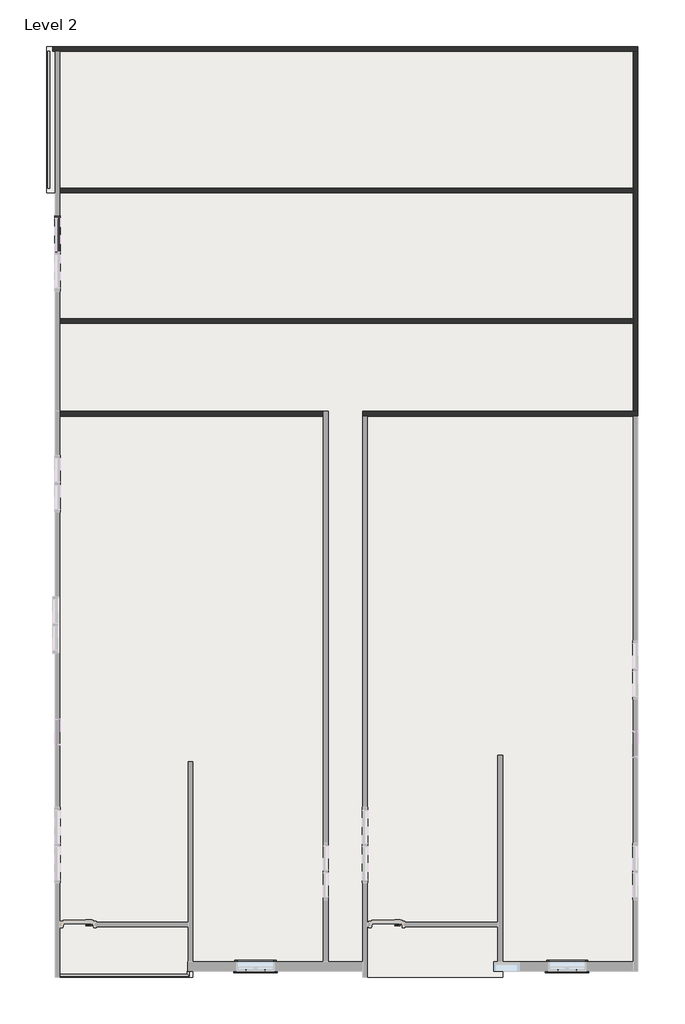
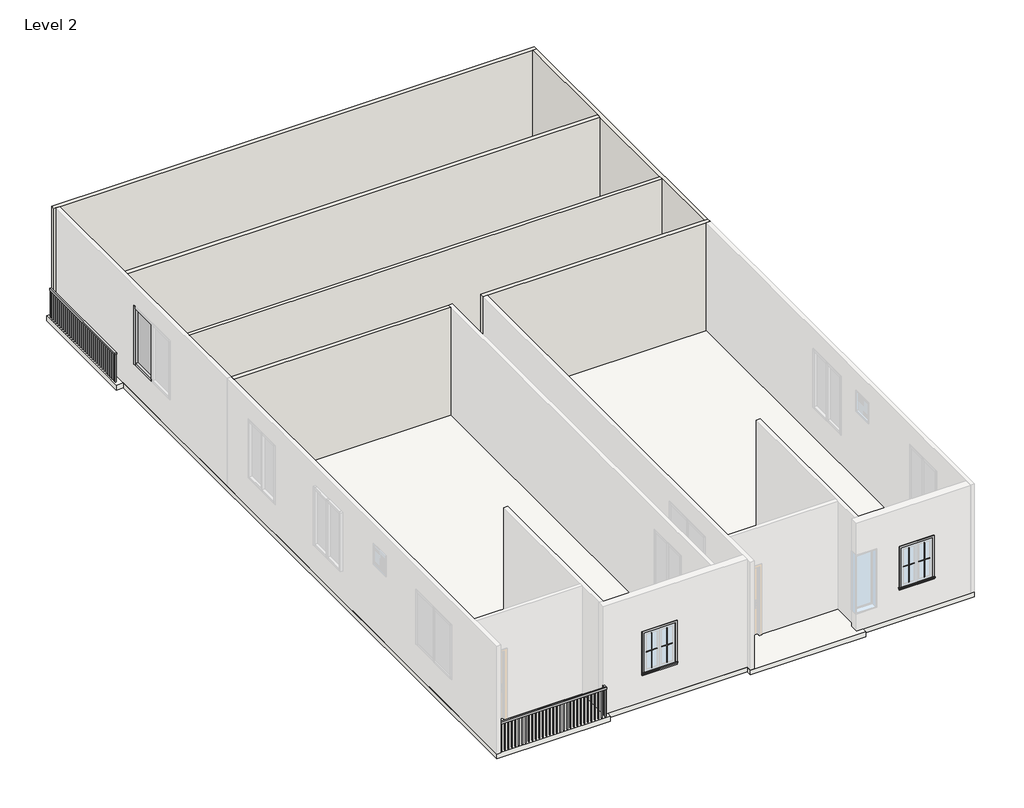
# One storey, part 2 of 2: 8 proxies, 6 walls, 3 railings, 2 members, 1 plate, 1 slab.
"""IFC4 building model written with IfcOpenShell, lengths in millimetres."""

from ifc_helpers import new_model, si_unit, frame, origin, place, context, project, spatial, polyline, outline, extrude, faceted_brep, transform, mapped, element, save
from components import muntin_pattern_2x2_muntin_pattern_2x2_1acec82f, muntin_pattern_2x2_muntin_pattern_2x2_43d02eee, trim_window_exterior_flat_with_sill_e4b28ec3, trim_window_interior_flat_picture_frame_39ff4276, member_2fae0574, member_3e1d4a65, system_panel_glazed_30879ba3

model = new_model("IFC4")

# Units and contexts
model_context = context("Model", 3, world=origin())
ifc_project = project(units=[si_unit("LENGTHUNIT", "METRE", prefix="MILLI")], contexts=[model_context])

# Site, building, storey
site = spatial("IfcSite", under=ifc_project)
building = spatial("IfcBuilding", under=site)
storey = spatial("IfcBuildingStorey", under=building, Name="Level 2", Elevation=3352.8)

# Proxies
placement = place(None, origin())
muntin_pattern_2x2_muntin_pattern_2x2_shape = muntin_pattern_2x2_muntin_pattern_2x2_1acec82f(model_context)
element("IfcBuildingElementProxy", 1, Name="Muntin Pattern_2x2 : Muntin Pattern_2x2", ObjectType="Muntin Pattern_2x2 : Muntin Pattern_2x2", at=placement, inside=storey, context=model_context, shape_type="MappedRepresentation", body=[
    mapped(muntin_pattern_2x2_muntin_pattern_2x2_shape, transform((-3129.6612038, -10576.3529557, 4337.05), x_axis=(-1.0, 0.0, 0.0), y_axis=(0.0, -1.0, 0.0), z_axis=(0.0, 0.0, 1.0))),
])
element("IfcBuildingElementProxy", 2, Name="Muntin Pattern_2x2 : Muntin Pattern_2x2", ObjectType="Muntin Pattern_2x2 : Muntin Pattern_2x2", at=placement, inside=storey, context=model_context, shape_type="MappedRepresentation", body=[
    mapped(muntin_pattern_2x2_muntin_pattern_2x2_shape, transform((4424.1833786, -10576.3529557, 4337.05), x_axis=(-1.0, 0.0, 0.0), y_axis=(0.0, -1.0, 0.0), z_axis=(0.0, 0.0, 1.0))),
])
muntin_pattern_2x2_muntin_pattern_2x2_2_shape = muntin_pattern_2x2_muntin_pattern_2x2_43d02eee(model_context)
element("IfcBuildingElementProxy", 3, Name="Muntin Pattern_2x2 : Muntin Pattern_2x2", ObjectType="Muntin Pattern_2x2 : Muntin Pattern_2x2", at=placement, inside=storey, context=model_context, shape_type="MappedRepresentation", body=[
    mapped(muntin_pattern_2x2_muntin_pattern_2x2_2_shape, transform((-3583.6862038, -10576.3529557, 4337.05), x_axis=(1.0, 0.0, 0.0), y_axis=(0.0, 1.0, 0.0), z_axis=(0.0, 0.0, 1.0))),
])
element("IfcBuildingElementProxy", 4, Name="Muntin Pattern_2x2 : Muntin Pattern_2x2", ObjectType="Muntin Pattern_2x2 : Muntin Pattern_2x2", at=placement, inside=storey, context=model_context, shape_type="MappedRepresentation", body=[
    mapped(muntin_pattern_2x2_muntin_pattern_2x2_2_shape, transform((3970.1583786, -10576.3529557, 4337.05), x_axis=(1.0, 0.0, 0.0), y_axis=(0.0, 1.0, 0.0), z_axis=(0.0, 0.0, 1.0))),
])
trim_window_exterior_flat_with_sill_shape = trim_window_exterior_flat_with_sill_e4b28ec3(model_context)
element("IfcBuildingElementProxy", 5, Name="Trim-Window-Exterior-Flat : with Sill", ObjectType="Trim-Window-Exterior-Flat : with Sill", at=placement, inside=storey, context=model_context, shape_type="MappedRepresentation", body=[
    mapped(trim_window_exterior_flat_with_sill_shape, transform((-3356.6737038, -10585.8779557, 5486.4), x_axis=(1.0, 0.0, 0.0), y_axis=(0.0, 0.0, 1.0), z_axis=(0.0, -1.0, 0.0))),
])
element("IfcBuildingElementProxy", 6, Name="Trim-Window-Exterior-Flat : with Sill", ObjectType="Trim-Window-Exterior-Flat : with Sill", at=placement, inside=storey, context=model_context, shape_type="MappedRepresentation", body=[
    mapped(trim_window_exterior_flat_with_sill_shape, transform((4197.1708786, -10585.8779557, 5486.4), x_axis=(1.0, 0.0, 0.0), y_axis=(0.0, 0.0, 1.0), z_axis=(0.0, -1.0, 0.0))),
])
trim_window_interior_flat_picture_frame_shape = trim_window_interior_flat_picture_frame_39ff4276(model_context)
element("IfcBuildingElementProxy", 7, Name="Trim-Window-Interior-Flat : Picture Frame", ObjectType="Trim-Window-Interior-Flat : Picture Frame", at=placement, inside=storey, context=model_context, shape_type="MappedRepresentation", body=[
    mapped(trim_window_interior_flat_picture_frame_shape, transform((-3356.6737038, -10357.2779557, 5486.4), x_axis=(-1.0, 0.0, 0.0), y_axis=(0.0, 0.0, 1.0), z_axis=(0.0, 1.0, 0.0))),
])
element("IfcBuildingElementProxy", 8, Name="Trim-Window-Interior-Flat : Picture Frame", ObjectType="Trim-Window-Interior-Flat : Picture Frame", at=placement, inside=storey, context=model_context, shape_type="MappedRepresentation", body=[
    mapped(trim_window_interior_flat_picture_frame_shape, transform((4197.1708786, -10357.2779557, 5486.4), x_axis=(-1.0, 0.0, 0.0), y_axis=(0.0, 0.0, 1.0), z_axis=(0.0, 1.0, 0.0))),
])

# Members
member_shape = member_2fae0574(model_context)
element("IfcMember", 9, ObjectType="Rectangular Mullion : 2.5\" x 5\" rectangular", at=placement, inside=storey, context=model_context, shape_type="MappedRepresentation", body=[
    mapped(member_shape, transform((-8153.157583, 7721.9533991, 6096.0), x_axis=(0.0, 1.0, 0.0), y_axis=(-1.0, 0.0, 0.0), z_axis=(0.0, 0.0, 1.0))),
])
member_2_shape = member_3e1d4a65(model_context)
element("IfcMember", 10, ObjectType="Rectangular Mullion : 2.5\" x 5\" rectangular", at=placement, inside=storey, context=model_context, shape_type="MappedRepresentation", body=[
    mapped(member_2_shape, transform((-8153.157583, 7658.4533991, 4267.2), x_axis=(0.0, 0.0, -1.0), y_axis=(-1.0, 0.0, 0.0), z_axis=(0.0, 1.0, 0.0))),
])

# Plate
system_panel_glazed_shape = system_panel_glazed_30879ba3(model_context)
element("IfcPlate", 11, ObjectType="System Panel : Glazed", at=placement, inside=storey, context=model_context, shape_type="MappedRepresentation", body=[
    mapped(system_panel_glazed_shape, transform((-8153.157583, 7248.6772692, 4330.7), x_axis=(0.0, -1.0, 0.0), y_axis=(1.0, 0.0, 0.0), z_axis=(0.0, 0.0, 1.0))),
])

# Railings
element("IfcRailing", 12, ObjectType="Handrail - Rectangular", at=placement, inside=storey, context=model_context, shape_type="SolidModel", body=[
    faceted_brep([(-8153.157583, -10659.0005933, 4267.2), (-8153.157583, -10659.0005933, 4216.4), (-8153.157583, -10709.8005933, 4216.4), (-8153.157583, -10709.8005933, 4267.2), (-5014.0237038, -10659.0005933, 4267.2), (-5014.0237038, -10659.0005933, 4216.4), (-4963.2237038, -10709.8005933, 4216.4), (-4963.2237038, -10709.8005933, 4267.2), (-5014.0237038, -10582.0742041, 4267.2), (-4963.2237038, -10582.0742041, 4267.2), (-4963.2237038, -10582.0742041, 4216.4), (-5014.0237038, -10582.0742041, 4216.4)], [[[0, 1, 2, 3]], [[1, 0, 4, 5]], [[2, 1, 5, 6]], [[3, 2, 6, 7]], [[0, 3, 7, 4]], [[8, 9, 10, 11]], [[5, 4, 8, 11]], [[6, 5, 11, 10]], [[7, 6, 10, 9]], [[4, 7, 9, 8]]]),
    extrude(outline(polyline([(-4979.0987038, -10592.3255933), (-4998.1487038, -10592.3255933), (-4998.1487038, -10573.2755933), (-4979.0987038, -10573.2755933), (-4979.0987038, -10592.3255933)])), frame((0.0, 0.0, 3352.8), z_axis=(0.0, 0.0, 1.0), x_axis=(1.0, 0.0, 0.0)), (0.0, 0.0, 1.0), 863.6),
    extrude(outline(polyline([(-5013.082583, -10693.9255933), (-5013.082583, -10674.8755933), (-4994.032583, -10674.8755933), (-4994.032583, -10693.9255933), (-5013.082583, -10693.9255933)])), frame((0.0, 0.0, 3352.8), z_axis=(0.0, 0.0, 1.0), x_axis=(1.0, 0.0, 0.0)), (0.0, 0.0, 1.0), 863.6),
    extrude(outline(polyline([(-5114.682583, -10693.9255933), (-5114.682583, -10674.8755933), (-5095.632583, -10674.8755933), (-5095.632583, -10693.9255933), (-5114.682583, -10693.9255933)])), frame((0.0, 0.0, 3352.8), z_axis=(0.0, 0.0, 1.0), x_axis=(1.0, 0.0, 0.0)), (0.0, 0.0, 1.0), 863.6),
    extrude(outline(polyline([(-5216.282583, -10693.9255933), (-5216.282583, -10674.8755933), (-5197.232583, -10674.8755933), (-5197.232583, -10693.9255933), (-5216.282583, -10693.9255933)])), frame((0.0, 0.0, 3352.8), z_axis=(0.0, 0.0, 1.0), x_axis=(1.0, 0.0, 0.0)), (0.0, 0.0, 1.0), 863.6),
    extrude(outline(polyline([(-5317.882583, -10693.9255933), (-5317.882583, -10674.8755933), (-5298.832583, -10674.8755933), (-5298.832583, -10693.9255933), (-5317.882583, -10693.9255933)])), frame((0.0, 0.0, 3352.8), z_axis=(0.0, 0.0, 1.0), x_axis=(1.0, 0.0, 0.0)), (0.0, 0.0, 1.0), 863.6),
    extrude(outline(polyline([(-5419.482583, -10693.9255933), (-5419.482583, -10674.8755933), (-5400.432583, -10674.8755933), (-5400.432583, -10693.9255933), (-5419.482583, -10693.9255933)])), frame((0.0, 0.0, 3352.8), z_axis=(0.0, 0.0, 1.0), x_axis=(1.0, 0.0, 0.0)), (0.0, 0.0, 1.0), 863.6),
    extrude(outline(polyline([(-5521.082583, -10693.9255933), (-5521.082583, -10674.8755933), (-5502.032583, -10674.8755933), (-5502.032583, -10693.9255933), (-5521.082583, -10693.9255933)])), frame((0.0, 0.0, 3352.8), z_axis=(0.0, 0.0, 1.0), x_axis=(1.0, 0.0, 0.0)), (0.0, 0.0, 1.0), 863.6),
    extrude(outline(polyline([(-5622.682583, -10693.9255933), (-5622.682583, -10674.8755933), (-5603.632583, -10674.8755933), (-5603.632583, -10693.9255933), (-5622.682583, -10693.9255933)])), frame((0.0, 0.0, 3352.8), z_axis=(0.0, 0.0, 1.0), x_axis=(1.0, 0.0, 0.0)), (0.0, 0.0, 1.0), 863.6),
    extrude(outline(polyline([(-5724.282583, -10693.9255933), (-5724.282583, -10674.8755933), (-5705.232583, -10674.8755933), (-5705.232583, -10693.9255933), (-5724.282583, -10693.9255933)])), frame((0.0, 0.0, 3352.8), z_axis=(0.0, 0.0, 1.0), x_axis=(1.0, 0.0, 0.0)), (0.0, 0.0, 1.0), 863.6),
    extrude(outline(polyline([(-5825.882583, -10693.9255933), (-5825.882583, -10674.8755933), (-5806.832583, -10674.8755933), (-5806.832583, -10693.9255933), (-5825.882583, -10693.9255933)])), frame((0.0, 0.0, 3352.8), z_axis=(0.0, 0.0, 1.0), x_axis=(1.0, 0.0, 0.0)), (0.0, 0.0, 1.0), 863.6),
    extrude(outline(polyline([(-5927.482583, -10693.9255933), (-5927.482583, -10674.8755933), (-5908.432583, -10674.8755933), (-5908.432583, -10693.9255933), (-5927.482583, -10693.9255933)])), frame((0.0, 0.0, 3352.8), z_axis=(0.0, 0.0, 1.0), x_axis=(1.0, 0.0, 0.0)), (0.0, 0.0, 1.0), 863.6),
    extrude(outline(polyline([(-6029.082583, -10693.9255933), (-6029.082583, -10674.8755933), (-6010.032583, -10674.8755933), (-6010.032583, -10693.9255933), (-6029.082583, -10693.9255933)])), frame((0.0, 0.0, 3352.8), z_axis=(0.0, 0.0, 1.0), x_axis=(1.0, 0.0, 0.0)), (0.0, 0.0, 1.0), 863.6),
    extrude(outline(polyline([(-6130.682583, -10693.9255933), (-6130.682583, -10674.8755933), (-6111.632583, -10674.8755933), (-6111.632583, -10693.9255933), (-6130.682583, -10693.9255933)])), frame((0.0, 0.0, 3352.8), z_axis=(0.0, 0.0, 1.0), x_axis=(1.0, 0.0, 0.0)), (0.0, 0.0, 1.0), 863.6),
    extrude(outline(polyline([(-6232.282583, -10693.9255933), (-6232.282583, -10674.8755933), (-6213.232583, -10674.8755933), (-6213.232583, -10693.9255933), (-6232.282583, -10693.9255933)])), frame((0.0, 0.0, 3352.8), z_axis=(0.0, 0.0, 1.0), x_axis=(1.0, 0.0, 0.0)), (0.0, 0.0, 1.0), 863.6),
    extrude(outline(polyline([(-6333.882583, -10693.9255933), (-6333.882583, -10674.8755933), (-6314.832583, -10674.8755933), (-6314.832583, -10693.9255933), (-6333.882583, -10693.9255933)])), frame((0.0, 0.0, 3352.8), z_axis=(0.0, 0.0, 1.0), x_axis=(1.0, 0.0, 0.0)), (0.0, 0.0, 1.0), 863.6),
    extrude(outline(polyline([(-6435.482583, -10693.9255933), (-6435.482583, -10674.8755933), (-6416.432583, -10674.8755933), (-6416.432583, -10693.9255933), (-6435.482583, -10693.9255933)])), frame((0.0, 0.0, 3352.8), z_axis=(0.0, 0.0, 1.0), x_axis=(1.0, 0.0, 0.0)), (0.0, 0.0, 1.0), 863.6),
    extrude(outline(polyline([(-6537.082583, -10693.9255933), (-6537.082583, -10674.8755933), (-6518.032583, -10674.8755933), (-6518.032583, -10693.9255933), (-6537.082583, -10693.9255933)])), frame((0.0, 0.0, 3352.8), z_axis=(0.0, 0.0, 1.0), x_axis=(1.0, 0.0, 0.0)), (0.0, 0.0, 1.0), 863.6),
    extrude(outline(polyline([(-6638.682583, -10693.9255933), (-6638.682583, -10674.8755933), (-6619.632583, -10674.8755933), (-6619.632583, -10693.9255933), (-6638.682583, -10693.9255933)])), frame((0.0, 0.0, 3352.8), z_axis=(0.0, 0.0, 1.0), x_axis=(1.0, 0.0, 0.0)), (0.0, 0.0, 1.0), 863.6),
    extrude(outline(polyline([(-6740.282583, -10693.9255933), (-6740.282583, -10674.8755933), (-6721.232583, -10674.8755933), (-6721.232583, -10693.9255933), (-6740.282583, -10693.9255933)])), frame((0.0, 0.0, 3352.8), z_axis=(0.0, 0.0, 1.0), x_axis=(1.0, 0.0, 0.0)), (0.0, 0.0, 1.0), 863.6),
    extrude(outline(polyline([(-6841.882583, -10693.9255933), (-6841.882583, -10674.8755933), (-6822.832583, -10674.8755933), (-6822.832583, -10693.9255933), (-6841.882583, -10693.9255933)])), frame((0.0, 0.0, 3352.8), z_axis=(0.0, 0.0, 1.0), x_axis=(1.0, 0.0, 0.0)), (0.0, 0.0, 1.0), 863.6),
    extrude(outline(polyline([(-6943.482583, -10693.9255933), (-6943.482583, -10674.8755933), (-6924.432583, -10674.8755933), (-6924.432583, -10693.9255933), (-6943.482583, -10693.9255933)])), frame((0.0, 0.0, 3352.8), z_axis=(0.0, 0.0, 1.0), x_axis=(1.0, 0.0, 0.0)), (0.0, 0.0, 1.0), 863.6),
    extrude(outline(polyline([(-7045.082583, -10693.9255933), (-7045.082583, -10674.8755933), (-7026.032583, -10674.8755933), (-7026.032583, -10693.9255933), (-7045.082583, -10693.9255933)])), frame((0.0, 0.0, 3352.8), z_axis=(0.0, 0.0, 1.0), x_axis=(1.0, 0.0, 0.0)), (0.0, 0.0, 1.0), 863.6),
    extrude(outline(polyline([(-7146.682583, -10693.9255933), (-7146.682583, -10674.8755933), (-7127.632583, -10674.8755933), (-7127.632583, -10693.9255933), (-7146.682583, -10693.9255933)])), frame((0.0, 0.0, 3352.8), z_axis=(0.0, 0.0, 1.0), x_axis=(1.0, 0.0, 0.0)), (0.0, 0.0, 1.0), 863.6),
    extrude(outline(polyline([(-7248.282583, -10693.9255933), (-7248.282583, -10674.8755933), (-7229.232583, -10674.8755933), (-7229.232583, -10693.9255933), (-7248.282583, -10693.9255933)])), frame((0.0, 0.0, 3352.8), z_axis=(0.0, 0.0, 1.0), x_axis=(1.0, 0.0, 0.0)), (0.0, 0.0, 1.0), 863.6),
    extrude(outline(polyline([(-7349.882583, -10693.9255933), (-7349.882583, -10674.8755933), (-7330.832583, -10674.8755933), (-7330.832583, -10693.9255933), (-7349.882583, -10693.9255933)])), frame((0.0, 0.0, 3352.8), z_axis=(0.0, 0.0, 1.0), x_axis=(1.0, 0.0, 0.0)), (0.0, 0.0, 1.0), 863.6),
    extrude(outline(polyline([(-7451.482583, -10693.9255933), (-7451.482583, -10674.8755933), (-7432.432583, -10674.8755933), (-7432.432583, -10693.9255933), (-7451.482583, -10693.9255933)])), frame((0.0, 0.0, 3352.8), z_axis=(0.0, 0.0, 1.0), x_axis=(1.0, 0.0, 0.0)), (0.0, 0.0, 1.0), 863.6),
    extrude(outline(polyline([(-7553.082583, -10693.9255933), (-7553.082583, -10674.8755933), (-7534.032583, -10674.8755933), (-7534.032583, -10693.9255933), (-7553.082583, -10693.9255933)])), frame((0.0, 0.0, 3352.8), z_axis=(0.0, 0.0, 1.0), x_axis=(1.0, 0.0, 0.0)), (0.0, 0.0, 1.0), 863.6),
    extrude(outline(polyline([(-7654.682583, -10693.9255933), (-7654.682583, -10674.8755933), (-7635.632583, -10674.8755933), (-7635.632583, -10693.9255933), (-7654.682583, -10693.9255933)])), frame((0.0, 0.0, 3352.8), z_axis=(0.0, 0.0, 1.0), x_axis=(1.0, 0.0, 0.0)), (0.0, 0.0, 1.0), 863.6),
    extrude(outline(polyline([(-7756.282583, -10693.9255933), (-7756.282583, -10674.8755933), (-7737.232583, -10674.8755933), (-7737.232583, -10693.9255933), (-7756.282583, -10693.9255933)])), frame((0.0, 0.0, 3352.8), z_axis=(0.0, 0.0, 1.0), x_axis=(1.0, 0.0, 0.0)), (0.0, 0.0, 1.0), 863.6),
    extrude(outline(polyline([(-7857.882583, -10693.9255933), (-7857.882583, -10674.8755933), (-7838.832583, -10674.8755933), (-7838.832583, -10693.9255933), (-7857.882583, -10693.9255933)])), frame((0.0, 0.0, 3352.8), z_axis=(0.0, 0.0, 1.0), x_axis=(1.0, 0.0, 0.0)), (0.0, 0.0, 1.0), 863.6),
    extrude(outline(polyline([(-7959.482583, -10693.9255933), (-7959.482583, -10674.8755933), (-7940.432583, -10674.8755933), (-7940.432583, -10693.9255933), (-7959.482583, -10693.9255933)])), frame((0.0, 0.0, 3352.8), z_axis=(0.0, 0.0, 1.0), x_axis=(1.0, 0.0, 0.0)), (0.0, 0.0, 1.0), 863.6),
    extrude(outline(polyline([(-8061.082583, -10693.9255933), (-8061.082583, -10674.8755933), (-8042.032583, -10674.8755933), (-8042.032583, -10693.9255933), (-8061.082583, -10693.9255933)])), frame((0.0, 0.0, 3352.8), z_axis=(0.0, 0.0, 1.0), x_axis=(1.0, 0.0, 0.0)), (0.0, 0.0, 1.0), 863.6),
    extrude(outline(polyline([(-4998.1487038, -10693.9255933), (-4998.1487038, -10674.8755933), (-4979.0987038, -10674.8755933), (-4979.0987038, -10693.9255933), (-4998.1487038, -10693.9255933)])), frame((0.0, 0.0, 3352.8), z_axis=(0.0, 0.0, 1.0), x_axis=(1.0, 0.0, 0.0)), (0.0, 0.0, 1.0), 863.6),
    extrude(outline(polyline([(-4979.0987038, -10601.1242041), (-4998.1487038, -10601.1242041), (-4998.1487038, -10582.0742041), (-4979.0987038, -10582.0742041), (-4979.0987038, -10601.1242041)])), frame((0.0, 0.0, 3352.8), z_axis=(0.0, 0.0, 1.0), x_axis=(1.0, 0.0, 0.0)), (0.0, 0.0, 1.0), 863.6),
    extrude(outline(polyline([(-8153.157583, -10693.9255933), (-8153.157583, -10674.8755933), (-8134.107583, -10674.8755933), (-8134.107583, -10693.9255933), (-8153.157583, -10693.9255933)])), frame((0.0, 0.0, 3352.8), z_axis=(0.0, 0.0, 1.0), x_axis=(1.0, 0.0, 0.0)), (0.0, 0.0, 1.0), 863.6),
])
element("IfcRailing", 13, ObjectType="Handrail - Rectangular", at=placement, inside=storey, context=model_context, shape_type="SweptSolid", body=[
    extrude(outline(polyline([(-8391.7551246, 11703.9189683), (-8340.9551246, 11703.9189683), (-8340.9551246, 8387.4224771), (-8391.7551246, 8387.4224771), (-8391.7551246, 11703.9189683)])), frame((0.0, 0.0, 4216.4), z_axis=(0.0, 0.0, 1.0), x_axis=(1.0, 0.0, 0.0)), (0.0, 0.0, 1.0), 50.8),
    extrude(outline(polyline([(-8375.8801246, 8462.2439683), (-8356.8301246, 8462.2439683), (-8356.8301246, 8443.1939683), (-8375.8801246, 8443.1939683), (-8375.8801246, 8462.2439683)])), frame((0.0, 0.0, 3352.8), z_axis=(0.0, 0.0, 1.0), x_axis=(1.0, 0.0, 0.0)), (0.0, 0.0, 1.0), 863.6),
    extrude(outline(polyline([(-8375.8801246, 8563.8439683), (-8356.8301246, 8563.8439683), (-8356.8301246, 8544.7939683), (-8375.8801246, 8544.7939683), (-8375.8801246, 8563.8439683)])), frame((0.0, 0.0, 3352.8), z_axis=(0.0, 0.0, 1.0), x_axis=(1.0, 0.0, 0.0)), (0.0, 0.0, 1.0), 863.6),
    extrude(outline(polyline([(-8375.8801246, 8665.4439683), (-8356.8301246, 8665.4439683), (-8356.8301246, 8646.3939683), (-8375.8801246, 8646.3939683), (-8375.8801246, 8665.4439683)])), frame((0.0, 0.0, 3352.8), z_axis=(0.0, 0.0, 1.0), x_axis=(1.0, 0.0, 0.0)), (0.0, 0.0, 1.0), 863.6),
    extrude(outline(polyline([(-8375.8801246, 8767.0439683), (-8356.8301246, 8767.0439683), (-8356.8301246, 8747.9939683), (-8375.8801246, 8747.9939683), (-8375.8801246, 8767.0439683)])), frame((0.0, 0.0, 3352.8), z_axis=(0.0, 0.0, 1.0), x_axis=(1.0, 0.0, 0.0)), (0.0, 0.0, 1.0), 863.6),
    extrude(outline(polyline([(-8375.8801246, 8868.6439683), (-8356.8301246, 8868.6439683), (-8356.8301246, 8849.5939683), (-8375.8801246, 8849.5939683), (-8375.8801246, 8868.6439683)])), frame((0.0, 0.0, 3352.8), z_axis=(0.0, 0.0, 1.0), x_axis=(1.0, 0.0, 0.0)), (0.0, 0.0, 1.0), 863.6),
    extrude(outline(polyline([(-8375.8801246, 8970.2439683), (-8356.8301246, 8970.2439683), (-8356.8301246, 8951.1939683), (-8375.8801246, 8951.1939683), (-8375.8801246, 8970.2439683)])), frame((0.0, 0.0, 3352.8), z_axis=(0.0, 0.0, 1.0), x_axis=(1.0, 0.0, 0.0)), (0.0, 0.0, 1.0), 863.6),
    extrude(outline(polyline([(-8375.8801246, 9071.8439683), (-8356.8301246, 9071.8439683), (-8356.8301246, 9052.7939683), (-8375.8801246, 9052.7939683), (-8375.8801246, 9071.8439683)])), frame((0.0, 0.0, 3352.8), z_axis=(0.0, 0.0, 1.0), x_axis=(1.0, 0.0, 0.0)), (0.0, 0.0, 1.0), 863.6),
    extrude(outline(polyline([(-8375.8801246, 9173.4439683), (-8356.8301246, 9173.4439683), (-8356.8301246, 9154.3939683), (-8375.8801246, 9154.3939683), (-8375.8801246, 9173.4439683)])), frame((0.0, 0.0, 3352.8), z_axis=(0.0, 0.0, 1.0), x_axis=(1.0, 0.0, 0.0)), (0.0, 0.0, 1.0), 863.6),
    extrude(outline(polyline([(-8375.8801246, 9275.0439683), (-8356.8301246, 9275.0439683), (-8356.8301246, 9255.9939683), (-8375.8801246, 9255.9939683), (-8375.8801246, 9275.0439683)])), frame((0.0, 0.0, 3352.8), z_axis=(0.0, 0.0, 1.0), x_axis=(1.0, 0.0, 0.0)), (0.0, 0.0, 1.0), 863.6),
    extrude(outline(polyline([(-8375.8801246, 9376.6439683), (-8356.8301246, 9376.6439683), (-8356.8301246, 9357.5939683), (-8375.8801246, 9357.5939683), (-8375.8801246, 9376.6439683)])), frame((0.0, 0.0, 3352.8), z_axis=(0.0, 0.0, 1.0), x_axis=(1.0, 0.0, 0.0)), (0.0, 0.0, 1.0), 863.6),
    extrude(outline(polyline([(-8375.8801246, 9478.2439683), (-8356.8301246, 9478.2439683), (-8356.8301246, 9459.1939683), (-8375.8801246, 9459.1939683), (-8375.8801246, 9478.2439683)])), frame((0.0, 0.0, 3352.8), z_axis=(0.0, 0.0, 1.0), x_axis=(1.0, 0.0, 0.0)), (0.0, 0.0, 1.0), 863.6),
    extrude(outline(polyline([(-8375.8801246, 9579.8439683), (-8356.8301246, 9579.8439683), (-8356.8301246, 9560.7939683), (-8375.8801246, 9560.7939683), (-8375.8801246, 9579.8439683)])), frame((0.0, 0.0, 3352.8), z_axis=(0.0, 0.0, 1.0), x_axis=(1.0, 0.0, 0.0)), (0.0, 0.0, 1.0), 863.6),
    extrude(outline(polyline([(-8375.8801246, 9681.4439683), (-8356.8301246, 9681.4439683), (-8356.8301246, 9662.3939683), (-8375.8801246, 9662.3939683), (-8375.8801246, 9681.4439683)])), frame((0.0, 0.0, 3352.8), z_axis=(0.0, 0.0, 1.0), x_axis=(1.0, 0.0, 0.0)), (0.0, 0.0, 1.0), 863.6),
    extrude(outline(polyline([(-8375.8801246, 9783.0439683), (-8356.8301246, 9783.0439683), (-8356.8301246, 9763.9939683), (-8375.8801246, 9763.9939683), (-8375.8801246, 9783.0439683)])), frame((0.0, 0.0, 3352.8), z_axis=(0.0, 0.0, 1.0), x_axis=(1.0, 0.0, 0.0)), (0.0, 0.0, 1.0), 863.6),
    extrude(outline(polyline([(-8375.8801246, 9884.6439683), (-8356.8301246, 9884.6439683), (-8356.8301246, 9865.5939683), (-8375.8801246, 9865.5939683), (-8375.8801246, 9884.6439683)])), frame((0.0, 0.0, 3352.8), z_axis=(0.0, 0.0, 1.0), x_axis=(1.0, 0.0, 0.0)), (0.0, 0.0, 1.0), 863.6),
    extrude(outline(polyline([(-8375.8801246, 9986.2439683), (-8356.8301246, 9986.2439683), (-8356.8301246, 9967.1939683), (-8375.8801246, 9967.1939683), (-8375.8801246, 9986.2439683)])), frame((0.0, 0.0, 3352.8), z_axis=(0.0, 0.0, 1.0), x_axis=(1.0, 0.0, 0.0)), (0.0, 0.0, 1.0), 863.6),
    extrude(outline(polyline([(-8375.8801246, 10087.8439683), (-8356.8301246, 10087.8439683), (-8356.8301246, 10068.7939683), (-8375.8801246, 10068.7939683), (-8375.8801246, 10087.8439683)])), frame((0.0, 0.0, 3352.8), z_axis=(0.0, 0.0, 1.0), x_axis=(1.0, 0.0, 0.0)), (0.0, 0.0, 1.0), 863.6),
    extrude(outline(polyline([(-8375.8801246, 10189.4439683), (-8356.8301246, 10189.4439683), (-8356.8301246, 10170.3939683), (-8375.8801246, 10170.3939683), (-8375.8801246, 10189.4439683)])), frame((0.0, 0.0, 3352.8), z_axis=(0.0, 0.0, 1.0), x_axis=(1.0, 0.0, 0.0)), (0.0, 0.0, 1.0), 863.6),
    extrude(outline(polyline([(-8375.8801246, 10291.0439683), (-8356.8301246, 10291.0439683), (-8356.8301246, 10271.9939683), (-8375.8801246, 10271.9939683), (-8375.8801246, 10291.0439683)])), frame((0.0, 0.0, 3352.8), z_axis=(0.0, 0.0, 1.0), x_axis=(1.0, 0.0, 0.0)), (0.0, 0.0, 1.0), 863.6),
    extrude(outline(polyline([(-8375.8801246, 10392.6439683), (-8356.8301246, 10392.6439683), (-8356.8301246, 10373.5939683), (-8375.8801246, 10373.5939683), (-8375.8801246, 10392.6439683)])), frame((0.0, 0.0, 3352.8), z_axis=(0.0, 0.0, 1.0), x_axis=(1.0, 0.0, 0.0)), (0.0, 0.0, 1.0), 863.6),
    extrude(outline(polyline([(-8375.8801246, 10494.2439683), (-8356.8301246, 10494.2439683), (-8356.8301246, 10475.1939683), (-8375.8801246, 10475.1939683), (-8375.8801246, 10494.2439683)])), frame((0.0, 0.0, 3352.8), z_axis=(0.0, 0.0, 1.0), x_axis=(1.0, 0.0, 0.0)), (0.0, 0.0, 1.0), 863.6),
    extrude(outline(polyline([(-8375.8801246, 10595.8439683), (-8356.8301246, 10595.8439683), (-8356.8301246, 10576.7939683), (-8375.8801246, 10576.7939683), (-8375.8801246, 10595.8439683)])), frame((0.0, 0.0, 3352.8), z_axis=(0.0, 0.0, 1.0), x_axis=(1.0, 0.0, 0.0)), (0.0, 0.0, 1.0), 863.6),
    extrude(outline(polyline([(-8375.8801246, 10697.4439683), (-8356.8301246, 10697.4439683), (-8356.8301246, 10678.3939683), (-8375.8801246, 10678.3939683), (-8375.8801246, 10697.4439683)])), frame((0.0, 0.0, 3352.8), z_axis=(0.0, 0.0, 1.0), x_axis=(1.0, 0.0, 0.0)), (0.0, 0.0, 1.0), 863.6),
    extrude(outline(polyline([(-8375.8801246, 10799.0439683), (-8356.8301246, 10799.0439683), (-8356.8301246, 10779.9939683), (-8375.8801246, 10779.9939683), (-8375.8801246, 10799.0439683)])), frame((0.0, 0.0, 3352.8), z_axis=(0.0, 0.0, 1.0), x_axis=(1.0, 0.0, 0.0)), (0.0, 0.0, 1.0), 863.6),
    extrude(outline(polyline([(-8375.8801246, 10900.6439683), (-8356.8301246, 10900.6439683), (-8356.8301246, 10881.5939683), (-8375.8801246, 10881.5939683), (-8375.8801246, 10900.6439683)])), frame((0.0, 0.0, 3352.8), z_axis=(0.0, 0.0, 1.0), x_axis=(1.0, 0.0, 0.0)), (0.0, 0.0, 1.0), 863.6),
    extrude(outline(polyline([(-8375.8801246, 11002.2439683), (-8356.8301246, 11002.2439683), (-8356.8301246, 10983.1939683), (-8375.8801246, 10983.1939683), (-8375.8801246, 11002.2439683)])), frame((0.0, 0.0, 3352.8), z_axis=(0.0, 0.0, 1.0), x_axis=(1.0, 0.0, 0.0)), (0.0, 0.0, 1.0), 863.6),
    extrude(outline(polyline([(-8375.8801246, 11103.8439683), (-8356.8301246, 11103.8439683), (-8356.8301246, 11084.7939683), (-8375.8801246, 11084.7939683), (-8375.8801246, 11103.8439683)])), frame((0.0, 0.0, 3352.8), z_axis=(0.0, 0.0, 1.0), x_axis=(1.0, 0.0, 0.0)), (0.0, 0.0, 1.0), 863.6),
    extrude(outline(polyline([(-8375.8801246, 11205.4439683), (-8356.8301246, 11205.4439683), (-8356.8301246, 11186.3939683), (-8375.8801246, 11186.3939683), (-8375.8801246, 11205.4439683)])), frame((0.0, 0.0, 3352.8), z_axis=(0.0, 0.0, 1.0), x_axis=(1.0, 0.0, 0.0)), (0.0, 0.0, 1.0), 863.6),
    extrude(outline(polyline([(-8375.8801246, 11307.0439683), (-8356.8301246, 11307.0439683), (-8356.8301246, 11287.9939683), (-8375.8801246, 11287.9939683), (-8375.8801246, 11307.0439683)])), frame((0.0, 0.0, 3352.8), z_axis=(0.0, 0.0, 1.0), x_axis=(1.0, 0.0, 0.0)), (0.0, 0.0, 1.0), 863.6),
    extrude(outline(polyline([(-8375.8801246, 11408.6439683), (-8356.8301246, 11408.6439683), (-8356.8301246, 11389.5939683), (-8375.8801246, 11389.5939683), (-8375.8801246, 11408.6439683)])), frame((0.0, 0.0, 3352.8), z_axis=(0.0, 0.0, 1.0), x_axis=(1.0, 0.0, 0.0)), (0.0, 0.0, 1.0), 863.6),
    extrude(outline(polyline([(-8375.8801246, 11510.2439683), (-8356.8301246, 11510.2439683), (-8356.8301246, 11491.1939683), (-8375.8801246, 11491.1939683), (-8375.8801246, 11510.2439683)])), frame((0.0, 0.0, 3352.8), z_axis=(0.0, 0.0, 1.0), x_axis=(1.0, 0.0, 0.0)), (0.0, 0.0, 1.0), 863.6),
    extrude(outline(polyline([(-8375.8801246, 11611.8439683), (-8356.8301246, 11611.8439683), (-8356.8301246, 11592.7939683), (-8375.8801246, 11592.7939683), (-8375.8801246, 11611.8439683)])), frame((0.0, 0.0, 3352.8), z_axis=(0.0, 0.0, 1.0), x_axis=(1.0, 0.0, 0.0)), (0.0, 0.0, 1.0), 863.6),
    extrude(outline(polyline([(-8375.8801246, 8406.4724771), (-8356.8301246, 8406.4724771), (-8356.8301246, 8387.4224771), (-8375.8801246, 8387.4224771), (-8375.8801246, 8406.4724771)])), frame((0.0, 0.0, 3352.8), z_axis=(0.0, 0.0, 1.0), x_axis=(1.0, 0.0, 0.0)), (0.0, 0.0, 1.0), 863.6),
    extrude(outline(polyline([(-8375.8801246, 11703.9189683), (-8356.8301246, 11703.9189683), (-8356.8301246, 11684.8689683), (-8375.8801246, 11684.8689683), (-8375.8801246, 11703.9189683)])), frame((0.0, 0.0, 3352.8), z_axis=(0.0, 0.0, 1.0), x_axis=(1.0, 0.0, 0.0)), (0.0, 0.0, 1.0), 863.6),
])
element("IfcRailing", 14, ObjectType="Handrail - Rectangular", at=placement, inside=storey, context=model_context, shape_type="SweptSolid", body=[
    extrude(outline(polyline([(5830.4721078, 11594.1725279), (5881.2721078, 11594.1725279), (5881.2721078, 8505.5262287), (5830.4721078, 8505.5262287), (5830.4721078, 11594.1725279)])), frame((0.0, 0.0, 4216.4), z_axis=(0.0, 0.0, 1.0), x_axis=(1.0, 0.0, 0.0)), (0.0, 0.0, 1.0), 50.8),
    extrude(outline(polyline([(5846.3471078, 8555.6975279), (5865.3971078, 8555.6975279), (5865.3971078, 8536.6475279), (5846.3471078, 8536.6475279), (5846.3471078, 8555.6975279)])), frame((0.0, 0.0, 3352.8), z_axis=(0.0, 0.0, 1.0), x_axis=(1.0, 0.0, 0.0)), (0.0, 0.0, 1.0), 863.6),
    extrude(outline(polyline([(5846.3471078, 8657.2975279), (5865.3971078, 8657.2975279), (5865.3971078, 8638.2475279), (5846.3471078, 8638.2475279), (5846.3471078, 8657.2975279)])), frame((0.0, 0.0, 3352.8), z_axis=(0.0, 0.0, 1.0), x_axis=(1.0, 0.0, 0.0)), (0.0, 0.0, 1.0), 863.6),
    extrude(outline(polyline([(5846.3471078, 8758.8975279), (5865.3971078, 8758.8975279), (5865.3971078, 8739.8475279), (5846.3471078, 8739.8475279), (5846.3471078, 8758.8975279)])), frame((0.0, 0.0, 3352.8), z_axis=(0.0, 0.0, 1.0), x_axis=(1.0, 0.0, 0.0)), (0.0, 0.0, 1.0), 863.6),
    extrude(outline(polyline([(5846.3471078, 8860.4975279), (5865.3971078, 8860.4975279), (5865.3971078, 8841.4475279), (5846.3471078, 8841.4475279), (5846.3471078, 8860.4975279)])), frame((0.0, 0.0, 3352.8), z_axis=(0.0, 0.0, 1.0), x_axis=(1.0, 0.0, 0.0)), (0.0, 0.0, 1.0), 863.6),
    extrude(outline(polyline([(5846.3471078, 8962.0975279), (5865.3971078, 8962.0975279), (5865.3971078, 8943.0475279), (5846.3471078, 8943.0475279), (5846.3471078, 8962.0975279)])), frame((0.0, 0.0, 3352.8), z_axis=(0.0, 0.0, 1.0), x_axis=(1.0, 0.0, 0.0)), (0.0, 0.0, 1.0), 863.6),
    extrude(outline(polyline([(5846.3471078, 9063.6975279), (5865.3971078, 9063.6975279), (5865.3971078, 9044.6475279), (5846.3471078, 9044.6475279), (5846.3471078, 9063.6975279)])), frame((0.0, 0.0, 3352.8), z_axis=(0.0, 0.0, 1.0), x_axis=(1.0, 0.0, 0.0)), (0.0, 0.0, 1.0), 863.6),
    extrude(outline(polyline([(5846.3471078, 9165.2975279), (5865.3971078, 9165.2975279), (5865.3971078, 9146.2475279), (5846.3471078, 9146.2475279), (5846.3471078, 9165.2975279)])), frame((0.0, 0.0, 3352.8), z_axis=(0.0, 0.0, 1.0), x_axis=(1.0, 0.0, 0.0)), (0.0, 0.0, 1.0), 863.6),
    extrude(outline(polyline([(5846.3471078, 9266.8975279), (5865.3971078, 9266.8975279), (5865.3971078, 9247.8475279), (5846.3471078, 9247.8475279), (5846.3471078, 9266.8975279)])), frame((0.0, 0.0, 3352.8), z_axis=(0.0, 0.0, 1.0), x_axis=(1.0, 0.0, 0.0)), (0.0, 0.0, 1.0), 863.6),
    extrude(outline(polyline([(5846.3471078, 9368.4975279), (5865.3971078, 9368.4975279), (5865.3971078, 9349.4475279), (5846.3471078, 9349.4475279), (5846.3471078, 9368.4975279)])), frame((0.0, 0.0, 3352.8), z_axis=(0.0, 0.0, 1.0), x_axis=(1.0, 0.0, 0.0)), (0.0, 0.0, 1.0), 863.6),
    extrude(outline(polyline([(5846.3471078, 9470.0975279), (5865.3971078, 9470.0975279), (5865.3971078, 9451.0475279), (5846.3471078, 9451.0475279), (5846.3471078, 9470.0975279)])), frame((0.0, 0.0, 3352.8), z_axis=(0.0, 0.0, 1.0), x_axis=(1.0, 0.0, 0.0)), (0.0, 0.0, 1.0), 863.6),
    extrude(outline(polyline([(5846.3471078, 9571.6975279), (5865.3971078, 9571.6975279), (5865.3971078, 9552.6475279), (5846.3471078, 9552.6475279), (5846.3471078, 9571.6975279)])), frame((0.0, 0.0, 3352.8), z_axis=(0.0, 0.0, 1.0), x_axis=(1.0, 0.0, 0.0)), (0.0, 0.0, 1.0), 863.6),
    extrude(outline(polyline([(5846.3471078, 9673.2975279), (5865.3971078, 9673.2975279), (5865.3971078, 9654.2475279), (5846.3471078, 9654.2475279), (5846.3471078, 9673.2975279)])), frame((0.0, 0.0, 3352.8), z_axis=(0.0, 0.0, 1.0), x_axis=(1.0, 0.0, 0.0)), (0.0, 0.0, 1.0), 863.6),
    extrude(outline(polyline([(5846.3471078, 9774.8975279), (5865.3971078, 9774.8975279), (5865.3971078, 9755.8475279), (5846.3471078, 9755.8475279), (5846.3471078, 9774.8975279)])), frame((0.0, 0.0, 3352.8), z_axis=(0.0, 0.0, 1.0), x_axis=(1.0, 0.0, 0.0)), (0.0, 0.0, 1.0), 863.6),
    extrude(outline(polyline([(5846.3471078, 9876.4975279), (5865.3971078, 9876.4975279), (5865.3971078, 9857.4475279), (5846.3471078, 9857.4475279), (5846.3471078, 9876.4975279)])), frame((0.0, 0.0, 3352.8), z_axis=(0.0, 0.0, 1.0), x_axis=(1.0, 0.0, 0.0)), (0.0, 0.0, 1.0), 863.6),
    extrude(outline(polyline([(5846.3471078, 9978.0975279), (5865.3971078, 9978.0975279), (5865.3971078, 9959.0475279), (5846.3471078, 9959.0475279), (5846.3471078, 9978.0975279)])), frame((0.0, 0.0, 3352.8), z_axis=(0.0, 0.0, 1.0), x_axis=(1.0, 0.0, 0.0)), (0.0, 0.0, 1.0), 863.6),
    extrude(outline(polyline([(5846.3471078, 10079.6975279), (5865.3971078, 10079.6975279), (5865.3971078, 10060.6475279), (5846.3471078, 10060.6475279), (5846.3471078, 10079.6975279)])), frame((0.0, 0.0, 3352.8), z_axis=(0.0, 0.0, 1.0), x_axis=(1.0, 0.0, 0.0)), (0.0, 0.0, 1.0), 863.6),
    extrude(outline(polyline([(5846.3471078, 10181.2975279), (5865.3971078, 10181.2975279), (5865.3971078, 10162.2475279), (5846.3471078, 10162.2475279), (5846.3471078, 10181.2975279)])), frame((0.0, 0.0, 3352.8), z_axis=(0.0, 0.0, 1.0), x_axis=(1.0, 0.0, 0.0)), (0.0, 0.0, 1.0), 863.6),
    extrude(outline(polyline([(5846.3471078, 10282.8975279), (5865.3971078, 10282.8975279), (5865.3971078, 10263.8475279), (5846.3471078, 10263.8475279), (5846.3471078, 10282.8975279)])), frame((0.0, 0.0, 3352.8), z_axis=(0.0, 0.0, 1.0), x_axis=(1.0, 0.0, 0.0)), (0.0, 0.0, 1.0), 863.6),
    extrude(outline(polyline([(5846.3471078, 10384.4975279), (5865.3971078, 10384.4975279), (5865.3971078, 10365.4475279), (5846.3471078, 10365.4475279), (5846.3471078, 10384.4975279)])), frame((0.0, 0.0, 3352.8), z_axis=(0.0, 0.0, 1.0), x_axis=(1.0, 0.0, 0.0)), (0.0, 0.0, 1.0), 863.6),
    extrude(outline(polyline([(5846.3471078, 10486.0975279), (5865.3971078, 10486.0975279), (5865.3971078, 10467.0475279), (5846.3471078, 10467.0475279), (5846.3471078, 10486.0975279)])), frame((0.0, 0.0, 3352.8), z_axis=(0.0, 0.0, 1.0), x_axis=(1.0, 0.0, 0.0)), (0.0, 0.0, 1.0), 863.6),
    extrude(outline(polyline([(5846.3471078, 10587.6975279), (5865.3971078, 10587.6975279), (5865.3971078, 10568.6475279), (5846.3471078, 10568.6475279), (5846.3471078, 10587.6975279)])), frame((0.0, 0.0, 3352.8), z_axis=(0.0, 0.0, 1.0), x_axis=(1.0, 0.0, 0.0)), (0.0, 0.0, 1.0), 863.6),
    extrude(outline(polyline([(5846.3471078, 10689.2975279), (5865.3971078, 10689.2975279), (5865.3971078, 10670.2475279), (5846.3471078, 10670.2475279), (5846.3471078, 10689.2975279)])), frame((0.0, 0.0, 3352.8), z_axis=(0.0, 0.0, 1.0), x_axis=(1.0, 0.0, 0.0)), (0.0, 0.0, 1.0), 863.6),
    extrude(outline(polyline([(5846.3471078, 10790.8975279), (5865.3971078, 10790.8975279), (5865.3971078, 10771.8475279), (5846.3471078, 10771.8475279), (5846.3471078, 10790.8975279)])), frame((0.0, 0.0, 3352.8), z_axis=(0.0, 0.0, 1.0), x_axis=(1.0, 0.0, 0.0)), (0.0, 0.0, 1.0), 863.6),
    extrude(outline(polyline([(5846.3471078, 10892.4975279), (5865.3971078, 10892.4975279), (5865.3971078, 10873.4475279), (5846.3471078, 10873.4475279), (5846.3471078, 10892.4975279)])), frame((0.0, 0.0, 3352.8), z_axis=(0.0, 0.0, 1.0), x_axis=(1.0, 0.0, 0.0)), (0.0, 0.0, 1.0), 863.6),
    extrude(outline(polyline([(5846.3471078, 10994.0975279), (5865.3971078, 10994.0975279), (5865.3971078, 10975.0475279), (5846.3471078, 10975.0475279), (5846.3471078, 10994.0975279)])), frame((0.0, 0.0, 3352.8), z_axis=(0.0, 0.0, 1.0), x_axis=(1.0, 0.0, 0.0)), (0.0, 0.0, 1.0), 863.6),
    extrude(outline(polyline([(5846.3471078, 11095.6975279), (5865.3971078, 11095.6975279), (5865.3971078, 11076.6475279), (5846.3471078, 11076.6475279), (5846.3471078, 11095.6975279)])), frame((0.0, 0.0, 3352.8), z_axis=(0.0, 0.0, 1.0), x_axis=(1.0, 0.0, 0.0)), (0.0, 0.0, 1.0), 863.6),
    extrude(outline(polyline([(5846.3471078, 11197.2975279), (5865.3971078, 11197.2975279), (5865.3971078, 11178.2475279), (5846.3471078, 11178.2475279), (5846.3471078, 11197.2975279)])), frame((0.0, 0.0, 3352.8), z_axis=(0.0, 0.0, 1.0), x_axis=(1.0, 0.0, 0.0)), (0.0, 0.0, 1.0), 863.6),
    extrude(outline(polyline([(5846.3471078, 11298.8975279), (5865.3971078, 11298.8975279), (5865.3971078, 11279.8475279), (5846.3471078, 11279.8475279), (5846.3471078, 11298.8975279)])), frame((0.0, 0.0, 3352.8), z_axis=(0.0, 0.0, 1.0), x_axis=(1.0, 0.0, 0.0)), (0.0, 0.0, 1.0), 863.6),
    extrude(outline(polyline([(5846.3471078, 11400.4975279), (5865.3971078, 11400.4975279), (5865.3971078, 11381.4475279), (5846.3471078, 11381.4475279), (5846.3471078, 11400.4975279)])), frame((0.0, 0.0, 3352.8), z_axis=(0.0, 0.0, 1.0), x_axis=(1.0, 0.0, 0.0)), (0.0, 0.0, 1.0), 863.6),
    extrude(outline(polyline([(5846.3471078, 11502.0975279), (5865.3971078, 11502.0975279), (5865.3971078, 11483.0475279), (5846.3471078, 11483.0475279), (5846.3471078, 11502.0975279)])), frame((0.0, 0.0, 3352.8), z_axis=(0.0, 0.0, 1.0), x_axis=(1.0, 0.0, 0.0)), (0.0, 0.0, 1.0), 863.6),
    extrude(outline(polyline([(5846.3471078, 8524.5762287), (5865.3971078, 8524.5762287), (5865.3971078, 8505.5262287), (5846.3471078, 8505.5262287), (5846.3471078, 8524.5762287)])), frame((0.0, 0.0, 3352.8), z_axis=(0.0, 0.0, 1.0), x_axis=(1.0, 0.0, 0.0)), (0.0, 0.0, 1.0), 863.6),
    extrude(outline(polyline([(5846.3471078, 11594.1725279), (5865.3971078, 11594.1725279), (5865.3971078, 11575.1225279), (5846.3471078, 11575.1225279), (5846.3471078, 11594.1725279)])), frame((0.0, 0.0, 3352.8), z_axis=(0.0, 0.0, 1.0), x_axis=(1.0, 0.0, 0.0)), (0.0, 0.0, 1.0), 863.6),
])

# Slab
element("IfcSlab", 15, ObjectType="6\" floor", at=placement, inside=storey, context=model_context, shape_type="SweptSolid", body=[
    extrude(outline(polyline([(5905.3208786, 11818.2189683), (5905.3208786, -10585.8779557), (2630.290751, -10585.8779557), (2630.290751, -10737.6531157), (-762.8431282, -10737.6531157), (-762.8431282, -10585.8779557), (-4874.3237038, -10585.8779557), (-4874.3237038, -10733.8493641), (-8210.307583, -10733.8493641), (-8210.307583, 8277.3011327), (-8419.607647, 8277.3011327), (-8419.607647, 11818.2189683), (5905.3208786, 11818.2189683)])), frame((0.0, 0.0, 3200.4), z_axis=(0.0, 0.0, 1.0), x_axis=(1.0, 0.0, 0.0)), (0.0, 0.0, 1.0), 152.4),
])

# Walls
element("IfcWall", 16, ObjectType="4.5\" wall", at=placement, inside=storey, context=model_context, shape_type="Brep", body=[
    faceted_brep([(-8267.457583, 11703.9189683, 3352.8), (-8210.307583, 11703.9189683, 3352.8), (-8096.007583, 11703.9189683, 3352.8), (5791.0208786, 11703.9189683, 3352.8), (5905.3208786, 11703.9189683, 3352.8), (5905.3208786, 11703.9189683, 6705.6), (5791.0208786, 11703.9189683, 6705.6), (-8096.007583, 11703.9189683, 6705.6), (-8210.307583, 11703.9189683, 6705.6), (-8267.457583, 11703.9189683, 6705.6), (-8267.457583, 11818.2189683, 3352.8), (-8267.457583, 11818.2189683, 6705.6), (5905.3208786, 11818.2189683, 6705.6), (5905.3208786, 11818.2189683, 3352.8)], [[[0, 1, 2, 3, 4, 5, 6, 7, 8, 9]], [[10, 11, 12, 13]], [[4, 3, 2, 1, 0, 10, 13]], [[9, 8, 7, 6, 5, 12, 11]], [[0, 9, 11, 10]], [[5, 4, 13, 12]]]),
])
element("IfcWall", 17, ObjectType="4.5\" wall", at=placement, inside=storey, context=model_context, shape_type="Brep", body=[
    faceted_brep([(5791.0208786, 11703.9189683, 3352.8), (5791.0208786, 8387.4224771, 3352.8), (5791.0208786, 8273.1224771, 3352.8), (5791.0208786, 5226.5048975, 3352.8), (5791.0208786, 5112.2048975, 3352.8), (5791.0208786, 2978.3002499, 3352.8), (5791.0208786, 2978.3002499, 6705.6), (5791.0208786, 5112.2048975, 6705.6), (5791.0208786, 5226.5048975, 6705.6), (5791.0208786, 8273.1224771, 6705.6), (5791.0208786, 8387.4224771, 6705.6), (5791.0208786, 11703.9189683, 6705.6), (5905.3208786, 11703.9189683, 3352.8), (5905.3208786, 11703.9189683, 6705.6), (5905.3208786, 2978.3002499, 6705.6), (5905.3208786, 2978.3002499, 3352.8)], [[[0, 1, 2, 3, 4, 5, 6, 7, 8, 9, 10, 11]], [[12, 13, 14, 15]], [[5, 4, 3, 2, 1, 0, 12, 15]], [[11, 10, 9, 8, 7, 6, 14, 13]], [[0, 11, 13, 12]], [[6, 5, 15, 14]]]),
])
element("IfcWall", 18, ObjectType="4.5\" wall", at=placement, inside=storey, context=model_context, shape_type="SweptSolid", body=[
    extrude(outline(polyline([(-1713.5935762, 2864.0002499), (-8096.007583, 2864.0002499), (-8096.007583, 2978.3002499), (-1713.5935762, 2978.3002499), (-1713.5935762, 2864.0002499)])), frame((0.0, 0.0, 3352.8), z_axis=(0.0, 0.0, 1.0), x_axis=(1.0, 0.0, 0.0)), (0.0, 0.0, 1.0), 3352.8),
])
element("IfcWall", 19, ObjectType="4.5\" wall", at=placement, inside=storey, context=model_context, shape_type="SweptSolid", body=[
    extrude(outline(polyline([(-8096.007583, 5226.5048975), (5791.0208786, 5226.5048975), (5791.0208786, 5112.2048975), (-8096.007583, 5112.2048975), (-8096.007583, 5226.5048975)])), frame((0.0, 0.0, 3352.8), z_axis=(0.0, 0.0, 1.0), x_axis=(1.0, 0.0, 0.0)), (0.0, 0.0, 1.0), 3352.8),
])
element("IfcWall", 20, ObjectType="4.5\" wall", at=placement, inside=storey, context=model_context, shape_type="SweptSolid", body=[
    extrude(outline(polyline([(-8096.007583, 8387.4224771), (5791.0208786, 8387.4224771), (5791.0208786, 8273.1224771), (-8096.007583, 8273.1224771), (-8096.007583, 8387.4224771)])), frame((0.0, 0.0, 3352.8), z_axis=(0.0, 0.0, 1.0), x_axis=(1.0, 0.0, 0.0)), (0.0, 0.0, 1.0), 3352.8),
])
element("IfcWall", 21, ObjectType="4.5\" wall", at=placement, inside=storey, context=model_context, shape_type="Brep", body=[
    faceted_brep([(-762.8431282, 2864.0002499, 3352.8), (-648.5431282, 2864.0002499, 3352.8), (5791.0208786, 2864.0002499, 3352.8), (5905.3208786, 2864.0002499, 3352.8), (5905.3208786, 2864.0002499, 6705.6), (5791.0208786, 2864.0002499, 6705.6), (-648.5431282, 2864.0002499, 6705.6), (-762.8431282, 2864.0002499, 6705.6), (-762.8431282, 2978.3002499, 3352.8), (-762.8431282, 2978.3002499, 6705.6), (5791.0208786, 2978.3002499, 6705.6), (5905.3208786, 2978.3002499, 6705.6), (5905.3208786, 2978.3002499, 3352.8), (5791.0208786, 2978.3002499, 3352.8)], [[[0, 1, 2, 3, 4, 5, 6, 7]], [[8, 9, 10, 11, 12, 13]], [[3, 2, 1, 0, 8, 13, 12]], [[7, 6, 5, 4, 11, 10, 9]], [[4, 3, 12, 11]], [[0, 7, 9, 8]]]),
])

save(model, "model.ifc")

# Revit data of these elements
# Type "Muntin Pattern_2x2 : Muntin Pattern_2x2"
#   Width [instance default] = 4' - 0"
#   Thickness = 0' - 0 1/2"
#   Height [instance default] = 4' - 0"
#   Distance = 0' - 0 3/4"
#   Interior Material [instance default] = none
#   Exterior Material [instance default] = none
#   Default Elevation = 0
# Type "Trim-Window-Exterior-Flat : with Sill"
#   Trim Width = 0' - 2 1/4"
#   Trim Thickness_Picture Frame = 0' - 1 1/4"
#   Trim Thickness_with Sill = 0' - 0 3/4"
#   Sill Thickness = 0' - 1 1/4"
#   Opening Width [instance default] = 2' - 0"
#   Opening Height [instance default] = 3' - 0"
#   Default Elevation = 4' - 0"
#   Sill = yes
#   Picture Frame = no
#   Trim Material [instance default] = none
# Type "Trim-Window-Interior-Flat : Picture Frame"
#   Trim Thickness_Picture Frame = 0' - 1 1/4"
#   Trim Width = 0' - 2 1/4"
#   Trim Thickness_with Sill = 0' - 0 3/4"
#   Sill Thickness = 0' - 1 1/4"
#   Opening Width [instance default] = 2' - 0"
#   Opening Height [instance default] = 3' - 0"
#   Default Elevation = 4' - 0"
#   Sill = no
#   Picture Frame = yes
#   Trim Material [instance default] = none
# Type "Rectangular Mullion : 2.5\" x 5\" rectangular"
#   built-in parameter 1007304 = 0.416667 (stored number, unit not read)
#   built-in parameter 1007301 = 0.104167 (stored number, unit not read)
#   built-in parameter 1007300 = 0.104167 (stored number, unit not read)
# Type "System Panel : Glazed"
#   Construction Type Id = "GSP4R"
#   Analytic Construction = "1/8 in Pilkington single glazing"
#   Visual Light Transmittance = 0.9
#   Solar Heat Gain Coefficient = 0.86
#   Heat Transfer Coefficient (U) = 1.18115 BTU/(h·ft²·°F)
#   Define Thermal Properties by = 1
# Type "Handrail - Rectangular"
#   Assembly Code = "C2010400"
#   built-in parameter 1008612 = 0.0416667 (stored number, unit not read)
#   built-in parameter 1008611 = 0.0416667 (stored number, unit not read)
#   built-in parameter 1008609 = 0.333333 (stored number, unit not read)
#   built-in parameter 1008604 = 0.166667 (stored number, unit not read)
#   built-in parameter 1008603 = 0.166667 (stored number, unit not read)
#   Railing Height = 3' - 0"
#   built-in parameter 1008630 = 2
#   built-in parameter 1008610 = 2
#   built-in parameter 1008618 = Baluster - Square : 3/4"
# Type "6\" floor"
#   Assembly Code = "B1010"
#   Function = 0
#   Layers, outside or top first: 0' - 6" no material (function 1)
# Type "4.5\" wall"
#   Assembly Code = "B2010"
#   Layers, outside or top first: 0' - 4 1/2" no material (function 1)
# Elements 1, 2, 3, 4 (IfcBuildingElementProxy, "Muntin Pattern_2x2 : Muntin Pattern_2x2")
#   Width = 1' - 0 5/8"
#   Height = 3' - 6 1/2"
#   Interior Material = Wood - Stained
#   Exterior Material = Clad - White
#   Phase Created = New Construction
#   Materials on its faces: "Clad - White", "Wood - Stained"
# Elements 5, 6 (IfcBuildingElementProxy, "Trim-Window-Exterior-Flat : with Sill")
#   Opening Width = 3' - 0"
#   Opening Height = 4' - 0"
#   Trim Material = Clad - White
#   Phase Created = New Construction
#   Materials on its faces: "Clad - White"
# Elements 7, 8 (IfcBuildingElementProxy, "Trim-Window-Interior-Flat : Picture Frame")
#   Opening Width = 3' - 0"
#   Opening Height = 4' - 0"
#   Trim Material = Wood - Stained
#   Phase Created = New Construction
#   Materials on its faces: "Wood - Stained"
# Elements 9, 10 (IfcMember, "Rectangular Mullion : 2.5\" x 5\" rectangular")
#   Phase Created = New Construction
#   Materials on its faces: "Aluminum"
# Element 11 (IfcPlate, "System Panel : Glazed")
#   Phase Created = New Construction
#   Materials on its faces: "Glass"
# Elements 12, 13, 14 (IfcRailing, "Handrail - Rectangular")
#   Phase Created = New Construction
# Element 15 (IfcSlab, "6\" floor")
#   Height Offset From Level = 0' - 0"
#   Phase Created = New Construction
#   Materials on its faces: "Default Floor"
# Elements 16, 17, 18, 19, 20, 21 (IfcWall, "4.5\" wall")
#   Top Offset = 0' - 0"
#   Base Offset = 0' - 0"
#   wall height = 11' - 0"
#   Phase Created = New Construction
#   Base Constraint = Level 2
#   Top Constraint = Level 3
#   Materials on its faces: "Default Wall"
# Materials
#   "Clad - White": class "Wood", colour RGB 242 242 238, transparency 0, Cost = 0
#   "Wood - Stained": class "Wood", colour RGB 224 178 126, transparency 0, Cost = 0
#   "Aluminum": class "Metal", colour RGB 247 247 247, transparency 0, Description = "Aluminum 6061", Cost = 0
#   "Glass": class "Glass", colour RGB 0 128 192, transparency 0.75, Description = "Soda Lime Glass", Cost = 0
#   "Default Floor": colour RGB 128 128 128, transparency 0, Cost = 0
#   "Default Wall": colour RGB 128 128 128, transparency 0, Cost = 0
